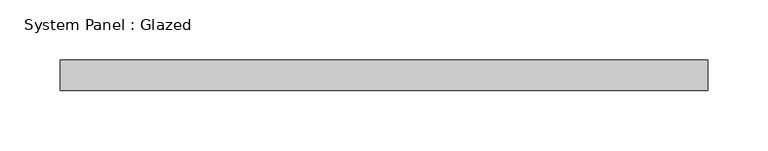
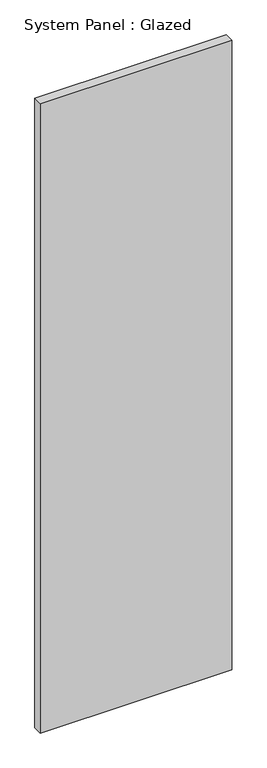
"""IFC4 building model written with IfcOpenShell, lengths in millimetres: plate geometry, System Panel : Glazed."""

from ifc_helpers import new_model, si_unit, origin, origin_with_axes, place, context, project, spatial, polyline, outline, extrude, source, transform, mapped, element, save


def system_panel_glazed_4b6d2a40(model_context):
    return source(origin(), model_context, "Body", "SweptSolid", [
        extrude(outline(polyline([(268.8166667, 19.05), (-268.8166667, 19.05), (-268.8166667, 44.45), (268.8166667, 44.45), (268.8166667, 19.05)])), origin_with_axes(), (0.0, 0.0, 1.0), 1868.867321),
    ])


if __name__ == "__main__":
    model = new_model("IFC4")
    model_context = context("Model", 3, world=origin())
    ifc_project = project(units=[si_unit("LENGTHUNIT", "METRE", prefix="MILLI")], contexts=[model_context])
    site = spatial("IfcSite", under=ifc_project)
    building = spatial("IfcBuilding", under=site)
    placement = place(None, origin())
    system_panel_glazed_shape = system_panel_glazed_4b6d2a40(model_context)
    element("IfcPlate", 1, ObjectType="System Panel : Glazed", at=placement, inside=building, context=model_context, shape_type="MappedRepresentation", body=[
        mapped(system_panel_glazed_shape, transform((0.0, 0.0, 0.0), x_axis=(1.0, 0.0, 0.0), y_axis=(0.0, 1.0, 0.0), z_axis=(0.0, 0.0, 1.0))),
    ])
    save(model, "model.ifc")

# Revit data of these elements
# Type "System Panel : Glazed"
#   Construction Type Id = "GSP4R"
#   Analytic Construction = "1/8 in Pilkington single glazing"
#   Visual Light Transmittance = 0.9
#   Solar Heat Gain Coefficient = 0.86
#   Heat Transfer Coefficient (U) = 1.18115 BTU/(h·ft²·°F)
#   Define Thermal Properties by = 1
# Element 1 (IfcPlate, "System Panel : Glazed")
#   Materials on its faces: "Glass"
# Materials
#   "Glass": class "Glass", colour RGB 0 128 192, transparency 0.75, Description = "Soda Lime Glass", Cost = 0
